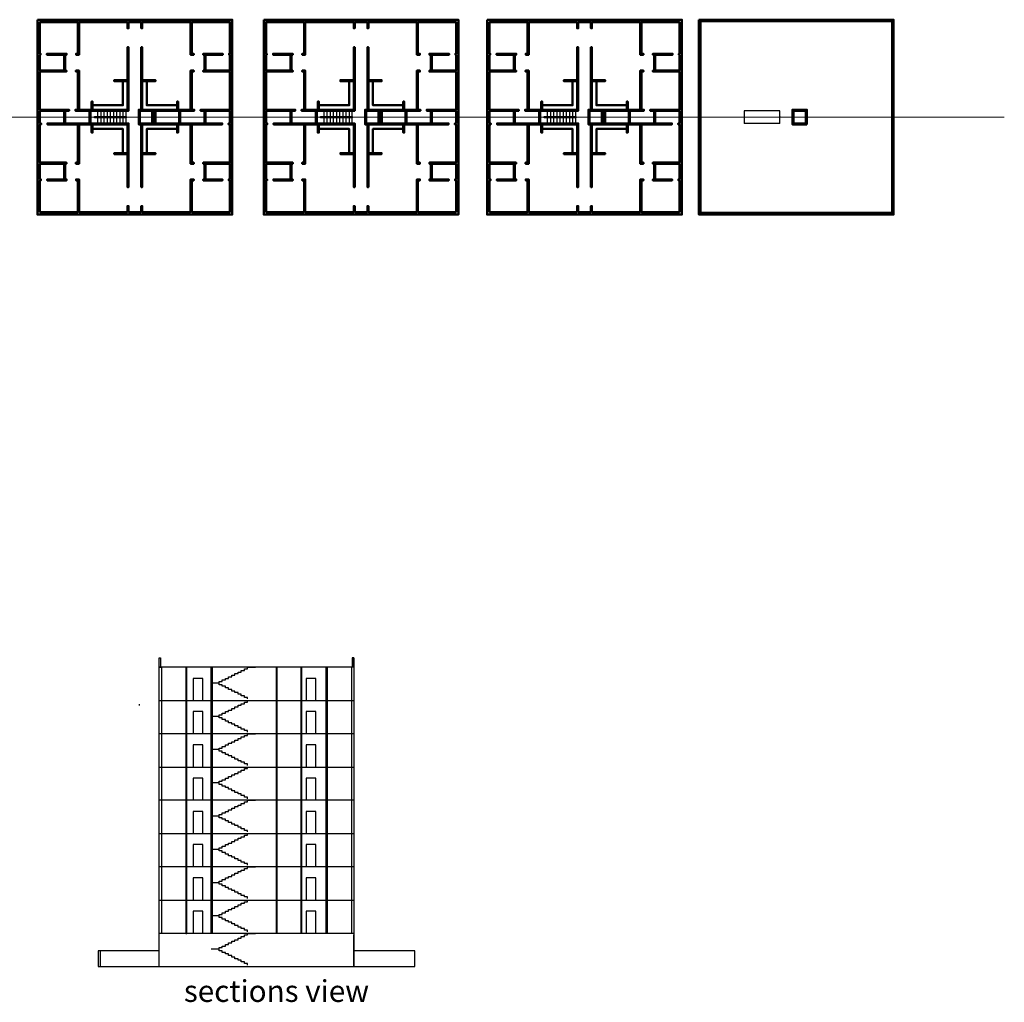
# Model space of a CAD drawing. Units: feet. Extents: x -1943 to 7856, y -1242 to 2749.
# Tile 2 of 2: x 4124 to 7856, y -1205 to 2518. Entities that reach past the tile are written whole.
import ezdxf

# ---------------------------------------------------------------- set-up
doc = ezdxf.new("R2010")
doc.units = ezdxf.units.FT
for name, color, linetype, lineweight in [('A-ANNO-SYMB', 1, 'Continuous', 18), ('A-ANNO-TEXT', 7, 'Continuous', 25), ('A-FLOR-STRS', 3, 'Continuous', 25), ('A-SECT', 7, 'Continuous', 25), ('A-WALL', 7, 'Continuous', 50)]:
    doc.layers.add(name, color=color, linetype=linetype, lineweight=lineweight)
doc.styles.get("Standard").update_dxf_attribs({"font": 'arial.ttf'})

# ---------------------------------------------------------------- blocks, each defined once
blk = doc.blocks.new('STAIR')
for p, q in [((-933.2, 2172.8), (-1068.1, 2172.8)), ((-1068.1, 2172.8), (-1068.1, 2124.8)), ((-1041.2, 2172.8), (-1041.2, 2151.4)), ((-1029.2, 2172.8), (-1029.2, 2151.4)), ((-1017.2, 2172.8), (-1017.2, 2151.4)), ((-1005.2, 2172.8), (-1005.2, 2151.4)), ((-993.2, 2172.8), (-993.2, 2151.4)), ((-981.2, 2172.8), (-981.2, 2151.4)), ((-969.2, 2172.8), (-969.2, 2151.4)), ((-957.2, 2172.8), (-957.2, 2151.4)), ((-945.2, 2172.8), (-945.2, 2151.4)), ((-1041.2, 2146.3), (-1041.2, 2124.8)), ((-1029.2, 2146.3), (-1029.2, 2124.8)), ((-1017.2, 2146.3), (-1017.2, 2124.8)), ((-1005.2, 2146.3), (-1005.2, 2124.8)), ((-993.2, 2146.3), (-993.2, 2124.8)), ((-981.2, 2146.3), (-981.2, 2124.8)), ((-969.2, 2146.3), (-969.2, 2124.8)), ((-957.2, 2146.3), (-957.2, 2124.8)), ((-933.2, 2124.8), (-1068.1, 2124.8))]:
    blk.add_line(p, q)
for points in [[(-933.2, 2124.8), (-933.2, 2172.8)], [(-945.2, 2146.3), (-945.2, 2124.8)]]:
    blk.add_lwpolyline(points)
for points in [[(-1053.2, 2151.4), (-933.2, 2151.4), (-933.2, 2146.3), (-1053.2, 2146.3)], [(-1052.2, 2150.4), (-934.2, 2150.4), (-934.2, 2147.3), (-1052.2, 2147.3)]]:
    blk.add_lwpolyline(points, close=True)

msp = doc.modelspace()

# ---------------------------------------------------------------- linework, layer by layer
at = {"layer": 'A-ANNO-SYMB'}
msp.add_line((-1942.9, 2148.8), (7856.1, 2148.8), dxfattribs=at)
at = {"layer": 'A-FLOR-STRS'}
for p, q in [((7005.2, 2172.8), (6870.3, 2172.8)), ((6870.3, 2172.8), (6870.3, 2124.8)), ((7005.2, 2124.8), (6870.3, 2124.8))]:
    msp.add_line(p, q, dxfattribs=at)
for points in [[(7005.2, 2124.8), (7005.2, 2172.8)], [(7005.2, 2151.4), (7005.2, 2148.8)]]:
    msp.add_lwpolyline(points, dxfattribs=at)
at = {"layer": 'A-SECT'}
for p, q in [((4652.5, 100.4), (4658.5, 100.4)), ((4652.5, -1069.6), (4652.5, 100.4)), ((4658.5, 100.4), (4658.5, 64.4)), ((5390.5, 100.4), (5384.5, 100.4)), ((5384.5, 100.4), (5384.5, 64.4)), ((5390.5, 64.4), (5390.5, 100.4)), ((5390.5, 100.4), (5390.5, -1069.6)), ((5390.5, 64.4), (4652.5, 64.4)), ((4652.5, 64.4), (4661.5, 64.4)), ((4661.5, 64.4), (4661.5, -943.6)), ((4753.5, 64.4), (4753.5, -943.6)), ((4757.5, -943.6), (4757.5, 64.4)), ((4849.5, -943.6), (4849.5, 64.4)), ((4849.5, 64.4), (4853.5, 64.4)), ((4853.5, 64.4), (4853.5, -943.6)), ((5100.7, 64.4), (5096.7, 64.4)), ((5096.7, 64.4), (5096.7, -943.6)), ((5100.7, -943.6), (5100.7, 64.4)), ((5189.5, 64.4), (5189.5, -943.6)), ((5193.5, -943.6), (5193.5, 64.4)), ((5285.5, -943.6), (5285.5, 64.4)), ((5289.5, 64.4), (5289.5, -943.6)), ((5381.5, 64.4), (5381.5, -943.6)), ((4652.5, -61.6), (5390.5, -61.6)), ((4577.1, -75.9, 316.9), (4577.1, -79.9, 316.9)), ((5390.5, -187.6), (4652.5, -187.6)), ((4652.5, -313.6), (5390.5, -313.6)), ((5390.5, -439.6), (4652.5, -439.6)), ((5390.5, -439.6), (4652.5, -439.6)), ((4652.5, -565.6), (5390.5, -565.6)), ((5390.5, -691.6), (4652.5, -691.6)), ((4652.5, -817.6), (5390.5, -817.6)), ((5390.5, -943.6), (4652.5, -943.6)), ((4753.5, -943.6), (4757.5, -943.6)), ((5390.5, -1069.6), (5390.5, -949.6)), ((4652.5, -1009.6), (4421.5, -1009.6)), ((4421.5, -1009.6), (4421.5, -1069.6)), ((4421.5, -1009.6), (4421.5, -1069.6)), ((4430.5, -1069.6), (4430.5, -1009.6)), ((5621.5, -1009.6), (5390.5, -1009.6)), ((5621.5, -1069.6), (5621.5, -1009.6)), ((4421.5, -1069.6), (5621.5, -1069.6))]:
    msp.add_line(p, q, dxfattribs=at)
for points in [[(4880.4, 4.4), (4880.4, 10.4), (4892.4, 10.4), (4892.4, 16.4), (4904.4, 16.4), (4904.4, 22.4), (4916.4, 22.4), (4916.4, 28.4), (4928.4, 28.4), (4928.4, 34.4), (4940.4, 34.4), (4940.4, 40.4), (4952.4, 40.4), (4952.4, 46.4), (4964.4, 46.4), (4964.4, 52.4), (4976.4, 52.4), (4976.4, 58.4), (4988.4, 58.4), (4988.4, 64.4), (5000.4, 64.4), (5018.5, 64.4)], [(4818.1, -61.6), (4818.1, 22.4), (4782.1, 22.4), (4782.1, -61.6)], [(4988.4, -55.6), (4988.4, -49.6), (4976.4, -49.6), (4976.4, -43.6), (4964.4, -43.6), (4964.4, -37.6), (4952.4, -37.6), (4952.4, -31.6), (4940.4, -31.6), (4940.4, -25.6), (4928.4, -25.6), (4928.4, -19.6), (4916.4, -19.6), (4916.4, -13.6), (4904.4, -13.6), (4904.4, -7.6), (4892.4, -7.6), (4892.4, -1.6), (4880.4, -1.6), (4880.4, 4.4), (4868.4, 4.4), (4850.4, 4.4)], [(5246.4, -61.6), (5246.4, 22.4), (5210.4, 22.4), (5210.4, -61.6)], [(4880.4, -121.6), (4880.4, -115.6), (4892.4, -115.6), (4892.4, -109.6), (4904.4, -109.6), (4904.4, -103.6), (4916.4, -103.6), (4916.4, -97.6), (4928.4, -97.6), (4928.4, -91.6), (4940.4, -91.6), (4940.4, -85.6), (4952.4, -85.6), (4952.4, -79.6), (4964.4, -79.6), (4964.4, -73.6), (4976.4, -73.6), (4976.4, -67.6), (4988.4, -67.6), (4988.4, -61.6), (5000.4, -61.6), (5018.5, -61.6)], [(4818.1, -187.6), (4818.1, -103.6), (4782.1, -103.6), (4782.1, -187.6)], [(5246.4, -187.6), (5246.4, -103.6), (5210.4, -103.6), (5210.4, -187.6)], [(4988.4, -181.6), (4988.4, -175.6), (4976.4, -175.6), (4976.4, -169.6), (4964.4, -169.6), (4964.4, -163.6), (4952.4, -163.6), (4952.4, -157.6), (4940.4, -157.6), (4940.4, -151.6), (4928.4, -151.6), (4928.4, -145.6), (4916.4, -145.6), (4916.4, -139.6), (4904.4, -139.6), (4904.4, -133.6), (4892.4, -133.6), (4892.4, -127.6), (4880.4, -127.6), (4880.4, -121.6), (4868.4, -121.6), (4850.4, -121.6)], [(4880.4, -247.6), (4880.4, -241.6), (4892.4, -241.6), (4892.4, -235.6), (4904.4, -235.6), (4904.4, -229.6), (4916.4, -229.6), (4916.4, -223.6), (4928.4, -223.6), (4928.4, -217.6), (4940.4, -217.6), (4940.4, -211.6), (4952.4, -211.6), (4952.4, -205.6), (4964.4, -205.6), (4964.4, -199.6), (4976.4, -199.6), (4976.4, -193.6), (4988.4, -193.6), (4988.4, -187.6), (5000.4, -187.6), (5018.5, -187.6)], [(4818.1, -313.6), (4818.1, -229.6), (4782.1, -229.6), (4782.1, -313.6)], [(4988.4, -307.6), (4988.4, -301.6), (4976.4, -301.6), (4976.4, -295.6), (4964.4, -295.6), (4964.4, -289.6), (4952.4, -289.6), (4952.4, -283.6), (4940.4, -283.6), (4940.4, -277.6), (4928.4, -277.6), (4928.4, -271.6), (4916.4, -271.6), (4916.4, -265.6), (4904.4, -265.6), (4904.4, -259.6), (4892.4, -259.6), (4892.4, -253.6), (4880.4, -253.6), (4880.4, -247.6), (4868.4, -247.6), (4850.4, -247.6)], [(5246.4, -313.6), (5246.4, -229.6), (5210.4, -229.6), (5210.4, -313.6)], [(4880.4, -373.6), (4880.4, -367.6), (4892.4, -367.6), (4892.4, -361.6), (4904.4, -361.6), (4904.4, -355.6), (4916.4, -355.6), (4916.4, -349.6), (4928.4, -349.6), (4928.4, -343.6), (4940.4, -343.6), (4940.4, -337.6), (4952.4, -337.6), (4952.4, -331.6), (4964.4, -331.6), (4964.4, -325.6), (4976.4, -325.6), (4976.4, -319.6), (4988.4, -319.6), (4988.4, -313.6), (5000.4, -313.6), (5018.5, -313.6)], [(4818.1, -439.6), (4818.1, -355.6), (4782.1, -355.6), (4782.1, -439.6)], [(5246.4, -439.6), (5246.4, -355.6), (5210.4, -355.6), (5210.4, -439.6)], [(4988.4, -433.6), (4988.4, -427.6), (4976.4, -427.6), (4976.4, -421.6), (4964.4, -421.6), (4964.4, -415.6), (4952.4, -415.6), (4952.4, -409.6), (4940.4, -409.6), (4940.4, -403.6), (4928.4, -403.6), (4928.4, -397.6), (4916.4, -397.6), (4916.4, -391.6), (4904.4, -391.6), (4904.4, -385.6), (4892.4, -385.6), (4892.4, -379.6), (4880.4, -379.6), (4880.4, -373.6), (4868.4, -373.6), (4850.4, -373.6)], [(4880.4, -499.6), (4880.4, -493.6), (4892.4, -493.6), (4892.4, -487.6), (4904.4, -487.6), (4904.4, -481.6), (4916.4, -481.6), (4916.4, -475.6), (4928.4, -475.6), (4928.4, -469.6), (4940.4, -469.6), (4940.4, -463.6), (4952.4, -463.6), (4952.4, -457.6), (4964.4, -457.6), (4964.4, -451.6), (4976.4, -451.6), (4976.4, -445.6), (4988.4, -445.6), (4988.4, -439.6), (5000.4, -439.6), (5018.5, -439.6)], [(4818.1, -565.6), (4818.1, -481.6), (4782.1, -481.6), (4782.1, -565.6)], [(5246.4, -565.6), (5246.4, -481.6), (5210.4, -481.6), (5210.4, -565.6)], [(4988.4, -559.6), (4988.4, -553.6), (4976.4, -553.6), (4976.4, -547.6), (4964.4, -547.6), (4964.4, -541.6), (4952.4, -541.6), (4952.4, -535.6), (4940.4, -535.6), (4940.4, -529.6), (4928.4, -529.6), (4928.4, -523.6), (4916.4, -523.6), (4916.4, -517.6), (4904.4, -517.6), (4904.4, -511.6), (4892.4, -511.6), (4892.4, -505.6), (4880.4, -505.6), (4880.4, -499.6), (4868.4, -499.6), (4850.4, -499.6)], [(4880.4, -625.6), (4880.4, -619.6), (4892.4, -619.6), (4892.4, -613.6), (4904.4, -613.6), (4904.4, -607.6), (4916.4, -607.6), (4916.4, -601.6), (4928.4, -601.6), (4928.4, -595.6), (4940.4, -595.6), (4940.4, -589.6), (4952.4, -589.6), (4952.4, -583.6), (4964.4, -583.6), (4964.4, -577.6), (4976.4, -577.6), (4976.4, -571.6), (4988.4, -571.6), (4988.4, -565.6), (5000.4, -565.6), (5018.5, -565.6)], [(4818.1, -691.6), (4818.1, -607.6), (4782.1, -607.6), (4782.1, -691.6)], [(4988.4, -685.6), (4988.4, -679.6), (4976.4, -679.6), (4976.4, -673.6), (4964.4, -673.6), (4964.4, -667.6), (4952.4, -667.6), (4952.4, -661.6), (4940.4, -661.6), (4940.4, -655.6), (4928.4, -655.6), (4928.4, -649.6), (4916.4, -649.6), (4916.4, -643.6), (4904.4, -643.6), (4904.4, -637.6), (4892.4, -637.6), (4892.4, -631.6), (4880.4, -631.6), (4880.4, -625.6), (4868.4, -625.6), (4850.4, -625.6)], [(5246.4, -691.6), (5246.4, -607.6), (5210.4, -607.6), (5210.4, -691.6)], [(4880.4, -751.6), (4880.4, -745.6), (4892.4, -745.6), (4892.4, -739.6), (4904.4, -739.6), (4904.4, -733.6), (4916.4, -733.6), (4916.4, -727.6), (4928.4, -727.6), (4928.4, -721.6), (4940.4, -721.6), (4940.4, -715.6), (4952.4, -715.6), (4952.4, -709.6), (4964.4, -709.6), (4964.4, -703.6), (4976.4, -703.6), (4976.4, -697.6), (4988.4, -697.6), (4988.4, -691.6), (5000.4, -691.6), (5018.5, -691.6)], [(4818.1, -817.6), (4818.1, -733.6), (4782.1, -733.6), (4782.1, -817.6)], [(5246.4, -817.6), (5246.4, -733.6), (5210.4, -733.6), (5210.4, -817.6)], [(4988.4, -811.6), (4988.4, -805.6), (4976.4, -805.6), (4976.4, -799.6), (4964.4, -799.6), (4964.4, -793.6), (4952.4, -793.6), (4952.4, -787.6), (4940.4, -787.6), (4940.4, -781.6), (4928.4, -781.6), (4928.4, -775.6), (4916.4, -775.6), (4916.4, -769.6), (4904.4, -769.6), (4904.4, -763.6), (4892.4, -763.6), (4892.4, -757.6), (4880.4, -757.6), (4880.4, -751.6), (4868.4, -751.6), (4850.4, -751.6)], [(4880.4, -877.6), (4880.4, -871.6), (4892.4, -871.6), (4892.4, -865.6), (4904.4, -865.6), (4904.4, -859.6), (4916.4, -859.6), (4916.4, -853.6), (4928.4, -853.6), (4928.4, -847.6), (4940.4, -847.6), (4940.4, -841.6), (4952.4, -841.6), (4952.4, -835.6), (4964.4, -835.6), (4964.4, -829.6), (4976.4, -829.6), (4976.4, -823.6), (4988.4, -823.6), (4988.4, -817.6), (5000.4, -817.6), (5018.5, -817.6)], [(4818.1, -943.6), (4818.1, -859.6), (4782.1, -859.6), (4782.1, -943.6)], [(4988.4, -937.6), (4988.4, -931.6), (4976.4, -931.6), (4976.4, -925.6), (4964.4, -925.6), (4964.4, -919.6), (4952.4, -919.6), (4952.4, -913.6), (4940.4, -913.6), (4940.4, -907.6), (4928.4, -907.6), (4928.4, -901.6), (4916.4, -901.6), (4916.4, -895.6), (4904.4, -895.6), (4904.4, -889.6), (4892.4, -889.6), (4892.4, -883.6), (4880.4, -883.6), (4880.4, -877.6), (4868.4, -877.6), (4850.4, -877.6)], [(5246.4, -943.6), (5246.4, -859.6), (5210.4, -859.6), (5210.4, -943.6)], [(4880.4, -1003.6), (4880.4, -997.6), (4892.4, -997.6), (4892.4, -991.6), (4904.4, -991.6), (4904.4, -985.6), (4916.4, -985.6), (4916.4, -979.6), (4928.4, -979.6), (4928.4, -973.6), (4940.4, -973.6), (4940.4, -967.6), (4952.4, -967.6), (4952.4, -961.6), (4964.4, -961.6), (4964.4, -955.6), (4976.4, -955.6), (4976.4, -949.6), (4988.4, -949.6), (4988.4, -943.6), (5000.4, -943.6), (5018.5, -943.6)], [(4988.4, -1063.6), (4988.4, -1057.6), (4976.4, -1057.6), (4976.4, -1051.6), (4964.4, -1051.6), (4964.4, -1045.6), (4952.4, -1045.6), (4952.4, -1039.6), (4940.4, -1039.6), (4940.4, -1033.6), (4928.4, -1033.6), (4928.4, -1027.6), (4916.4, -1027.6), (4916.4, -1021.6), (4904.4, -1021.6), (4904.4, -1015.6), (4892.4, -1015.6), (4892.4, -1009.6), (4880.4, -1009.6), (4880.4, -1003.6), (4868.4, -1003.6), (4850.4, -1003.6)]]:
    msp.add_lwpolyline(points, dxfattribs=at)
at = {"layer": 'A-WALL'}
for p, q in [((4639, 2288.8), (4639, 2288.8)), ((5496.3, 2288.8), (5496.3, 2288.8)), ((6343.2, 2288.8), (6343.2, 2288.8))]:
    msp.add_line(p, q, dxfattribs=at)
for points in [[(4191.9, 2517.8), (4191.9, 1779.8), (4929.9, 1779.8), (4929.9, 2517.8)], [(5049.2, 2517.8), (5049.2, 1779.8), (5787.2, 1779.8), (5787.2, 2517.8)], [(5896.1, 2517.8), (5896.1, 1779.8), (6634.1, 1779.8), (6634.1, 2517.8)], [(6698.6, 2517.8), (6698.6, 1779.8), (7436.6, 1779.8), (7436.6, 2517.8)], [(6704.6, 2511.8), (6704.6, 1785.8), (7430.6, 1785.8), (7430.6, 2511.8)], [(4630.5, 2120.8), (4575.8, 2120.8), (4575.8, 2176.8), (4630.5, 2176.8)], [(4626.5, 2124.8), (4579.8, 2124.8), (4579.8, 2172.8), (4626.5, 2172.8)], [(5487.8, 2120.8), (5433.2, 2120.8), (5433.2, 2176.8), (5487.8, 2176.8)], [(5483.8, 2124.8), (5437.2, 2124.8), (5437.2, 2172.8), (5483.8, 2172.8)], [(6334.7, 2120.8), (6280.1, 2120.8), (6280.1, 2176.8), (6334.7, 2176.8)], [(6330.7, 2124.8), (6284.1, 2124.8), (6284.1, 2172.8), (6330.7, 2172.8)], [(7107.8, 2120.8), (7053.2, 2120.8), (7053.2, 2176.8), (7107.8, 2176.8)], [(7103.8, 2124.8), (7057.2, 2124.8), (7057.2, 2172.8), (7103.8, 2172.8)]]:
    msp.add_lwpolyline(points, close=True, dxfattribs=at)
for points in [[(4732.9, 2124.8), (4824.9, 2124.8), (4824.9, 2172.8), (4810, 2172.8), (4810, 2176.8), (4920.9, 2176.8), (4920.9, 2321.3), (4820.1, 2321.3), (4820.1, 2325.3), (4824.9, 2325.3), (4824.9, 2384.8), (4819.8, 2384.8), (4819.8, 2388.8), (4894.3, 2388.8), (4894.3, 2384.8), (4828.9, 2384.8), (4828.9, 2325.3), (4920.9, 2325.3), (4920.9, 2384.8), (4918.3, 2384.8), (4918.3, 2388.8), (4920.9, 2388.8), (4920.9, 2508.8), (4776.4, 2508.8), (4776.4, 2388.8), (4783.8, 2388.8), (4783.8, 2384.8), (4772.4, 2384.8), (4772.4, 2508.8), (4588.9, 2508.8), (4588.9, 2485.7), (4584.9, 2485.7), (4584.9, 2508.8), (4536.9, 2508.8), (4536.9, 2485.7), (4532.9, 2485.7), (4532.9, 2508.8), (4349.4, 2508.8), (4349.4, 2384.8), (4337.9, 2384.8), (4337.9, 2388.8), (4345.4, 2388.8), (4345.4, 2508.8), (4200.9, 2508.8), (4200.9, 2388.8), (4203.4, 2388.8), (4203.4, 2384.8), (4200.9, 2384.8), (4200.9, 2325.3), (4292.9, 2325.3), (4292.9, 2384.8), (4227.4, 2384.8), (4227.4, 2388.8), (4301.9, 2388.8), (4301.9, 2384.8), (4296.9, 2384.8), (4296.9, 2325.3), (4301.7, 2325.3), (4301.7, 2321.3), (4200.9, 2321.3), (4200.9, 2176.8), (4311.8, 2176.8), (4311.8, 2172.8), (4296.9, 2172.8), (4296.9, 2124.8), (4388.9, 2124.8), (4388.9, 2172.8), (4388.9, 2124.8), (4388.9, 2172.8), (4335.8, 2172.8), (4335.8, 2176.8), (4345.4, 2176.8), (4345.4, 2321.3), (4337.7, 2321.3), (4337.7, 2325.3), (4349.4, 2325.3), (4349.4, 2176.8), (4396.9, 2176.8), (4396.9, 2207.4), (4400.9, 2207.4), (4400.9, 2176.8), (4532.9, 2176.8), (4532.9, 2284.8), (4482.8, 2284.8), (4482.8, 2288.8), (4532.9, 2288.8), (4532.9, 2413.7), (4536.9, 2413.7), (4536.9, 2172.8), (4392.9, 2172.8), (4392.9, 2124.8), (4536.9, 2124.8), (4536.9, 1884), (4532.9, 1884), (4532.9, 2008.8), (4482.8, 2008.8), (4482.8, 2012.8), (4532.9, 2012.8), (4532.9, 2120.8), (4400.9, 2120.8), (4400.9, 2090.3), (4396.9, 2090.3), (4396.9, 2120.8), (4349.4, 2120.8), (4349.4, 1972.3), (4337.7, 1972.3), (4337.7, 1976.3), (4345.4, 1976.3), (4345.4, 2120.8), (4229.4, 2120.8), (4229.4, 2124.8), (4292.9, 2124.8), (4292.9, 2172.8), (4200.9, 2172.8), (4200.9, 2124.8), (4205.4, 2124.8), (4205.4, 2120.8), (4200.9, 2120.8), (4200.9, 1976.3), (4301.7, 1976.3), (4301.7, 1972.3), (4296.9, 1972.3), (4296.9, 1912.8), (4301.9, 1912.8), (4301.9, 1908.8), (4228.8, 1908.8), (4228.8, 1912.8), (4292.9, 1912.8), (4292.9, 1972.3), (4200.9, 1972.3), (4200.9, 1912.8), (4204.8, 1912.8), (4204.8, 1908.8), (4200.9, 1908.8), (4200.9, 1788.8), (4345.4, 1788.8), (4345.4, 1908.8), (4337.9, 1908.8), (4337.9, 1912.8), (4349.4, 1912.8), (4349.4, 1788.8), (4532.9, 1788.8), (4532.9, 1812), (4536.9, 1812), (4536.9, 1788.8), (4584.9, 1788.8), (4584.9, 1812), (4588.9, 1812), (4588.9, 1788.8), (4772.4, 1788.8), (4772.4, 1912.8), (4783.8, 1912.8), (4783.8, 1908.8), (4776.4, 1908.8), (4776.4, 1788.8), (4920.9, 1788.8), (4920.9, 1908.8), (4917, 1908.8), (4917, 1912.8), (4920.9, 1912.8), (4920.9, 1972.3), (4828.9, 1972.3), (4828.9, 1912.8), (4893, 1912.8), (4893, 1908.8), (4819.8, 1908.8), (4819.8, 1912.8), (4824.9, 1912.8), (4824.9, 1972.3), (4820.1, 1972.3), (4820.1, 1976.3), (4920.9, 1976.3), (4920.9, 2120.8), (4916.4, 2120.8), (4916.4, 2124.8), (4920.9, 2124.8), (4920.9, 2172.8), (4828.9, 2172.8), (4828.9, 2124.8), (4892.4, 2124.8), (4892.4, 2120.8), (4776.4, 2120.8), (4776.4, 1976.3), (4784.1, 1976.3), (4784.1, 1972.3), (4772.4, 1972.3), (4772.4, 2120.8), (4724.9, 2120.8), (4724.9, 2090.3), (4720.9, 2090.3), (4720.9, 2120.8), (4588.9, 2120.8), (4588.9, 2012.8), (4639, 2012.8), (4639, 2008.8), (4588.9, 2008.8), (4588.9, 1884), (4584.9, 1884), (4584.9, 2124.8), (4635.5, 2124.8), (4635.5, 2172.8), (4584.9, 2172.8), (4584.9, 2413.7), (4588.9, 2413.7), (4588.9, 2288.8), (4639, 2288.8), (4639, 2284.8), (4588.9, 2284.8), (4588.9, 2176.8), (4720.9, 2176.8), (4720.9, 2207.4), (4724.9, 2207.4), (4724.9, 2176.8), (4772.4, 2176.8), (4772.4, 2325.3), (4784.1, 2325.3), (4784.1, 2321.3), (4776.4, 2321.3), (4776.4, 2176.8), (4786, 2176.8), (4786, 2172.8), (4732.9, 2172.8), (4732.9, 2124.8), (4732.9, 2172.8)], [(5590.2, 2124.8), (5682.2, 2124.8), (5682.2, 2172.8), (5667.3, 2172.8), (5667.3, 2176.8), (5778.2, 2176.8), (5778.2, 2321.3), (5677.4, 2321.3), (5677.4, 2325.3), (5682.2, 2325.3), (5682.2, 2384.8), (5677.2, 2384.8), (5677.2, 2388.8), (5751.7, 2388.8), (5751.7, 2384.8), (5686.2, 2384.8), (5686.2, 2325.3), (5778.2, 2325.3), (5778.2, 2384.8), (5775.7, 2384.8), (5775.7, 2388.8), (5778.2, 2388.8), (5778.2, 2508.8), (5633.7, 2508.8), (5633.7, 2388.8), (5641.2, 2388.8), (5641.2, 2384.8), (5629.7, 2384.8), (5629.7, 2508.8), (5446.2, 2508.8), (5446.2, 2485.7), (5442.2, 2485.7), (5442.2, 2508.8), (5394.2, 2508.8), (5394.2, 2485.7), (5390.2, 2485.7), (5390.2, 2508.8), (5206.7, 2508.8), (5206.7, 2384.8), (5195.3, 2384.8), (5195.3, 2388.8), (5202.7, 2388.8), (5202.7, 2508.8), (5058.2, 2508.8), (5058.2, 2388.8), (5060.8, 2388.8), (5060.8, 2384.8), (5058.2, 2384.8), (5058.2, 2325.3), (5150.2, 2325.3), (5150.2, 2384.8), (5084.8, 2384.8), (5084.8, 2388.8), (5159.3, 2388.8), (5159.3, 2384.8), (5154.2, 2384.8), (5154.2, 2325.3), (5159.1, 2325.3), (5159.1, 2321.3), (5058.2, 2321.3), (5058.2, 2176.8), (5169.1, 2176.8), (5169.1, 2172.8), (5154.2, 2172.8), (5154.2, 2124.8), (5246.2, 2124.8), (5246.2, 2172.8), (5246.2, 2124.8), (5246.2, 2172.8), (5193.1, 2172.8), (5193.1, 2176.8), (5202.7, 2176.8), (5202.7, 2321.3), (5195.1, 2321.3), (5195.1, 2325.3), (5206.7, 2325.3), (5206.7, 2176.8), (5254.2, 2176.8), (5254.2, 2207.4), (5258.2, 2207.4), (5258.2, 2176.8), (5390.2, 2176.8), (5390.2, 2284.8), (5340.2, 2284.8), (5340.2, 2288.8), (5390.2, 2288.8), (5390.2, 2413.7), (5394.2, 2413.7), (5394.2, 2172.8), (5250.2, 2172.8), (5250.2, 2124.8), (5394.2, 2124.8), (5394.2, 1884), (5390.2, 1884), (5390.2, 2008.8), (5340.2, 2008.8), (5340.2, 2012.8), (5390.2, 2012.8), (5390.2, 2120.8), (5258.2, 2120.8), (5258.2, 2090.3), (5254.2, 2090.3), (5254.2, 2120.8), (5206.7, 2120.8), (5206.7, 1972.3), (5195.1, 1972.3), (5195.1, 1976.3), (5202.7, 1976.3), (5202.7, 2120.8), (5086.7, 2120.8), (5086.7, 2124.8), (5150.2, 2124.8), (5150.2, 2172.8), (5058.2, 2172.8), (5058.2, 2124.8), (5062.7, 2124.8), (5062.7, 2120.8), (5058.2, 2120.8), (5058.2, 1976.3), (5159.1, 1976.3), (5159.1, 1972.3), (5154.2, 1972.3), (5154.2, 1912.8), (5159.3, 1912.8), (5159.3, 1908.8), (5086.1, 1908.8), (5086.1, 1912.8), (5150.2, 1912.8), (5150.2, 1972.3), (5058.2, 1972.3), (5058.2, 1912.8), (5062.1, 1912.8), (5062.1, 1908.8), (5058.2, 1908.8), (5058.2, 1788.8), (5202.7, 1788.8), (5202.7, 1908.8), (5195.3, 1908.8), (5195.3, 1912.8), (5206.7, 1912.8), (5206.7, 1788.8), (5390.2, 1788.8), (5390.2, 1812), (5394.2, 1812), (5394.2, 1788.8), (5442.2, 1788.8), (5442.2, 1812), (5446.2, 1812), (5446.2, 1788.8), (5629.7, 1788.8), (5629.7, 1912.8), (5641.2, 1912.8), (5641.2, 1908.8), (5633.7, 1908.8), (5633.7, 1788.8), (5778.2, 1788.8), (5778.2, 1908.8), (5774.3, 1908.8), (5774.3, 1912.8), (5778.2, 1912.8), (5778.2, 1972.3), (5686.2, 1972.3), (5686.2, 1912.8), (5750.3, 1912.8), (5750.3, 1908.8), (5677.2, 1908.8), (5677.2, 1912.8), (5682.2, 1912.8), (5682.2, 1972.3), (5677.4, 1972.3), (5677.4, 1976.3), (5778.2, 1976.3), (5778.2, 2120.8), (5773.7, 2120.8), (5773.7, 2124.8), (5778.2, 2124.8), (5778.2, 2172.8), (5686.2, 2172.8), (5686.2, 2124.8), (5749.7, 2124.8), (5749.7, 2120.8), (5633.7, 2120.8), (5633.7, 1976.3), (5641.4, 1976.3), (5641.4, 1972.3), (5629.7, 1972.3), (5629.7, 2120.8), (5582.2, 2120.8), (5582.2, 2090.3), (5578.2, 2090.3), (5578.2, 2120.8), (5446.2, 2120.8), (5446.2, 2012.8), (5496.3, 2012.8), (5496.3, 2008.8), (5446.2, 2008.8), (5446.2, 1884), (5442.2, 1884), (5442.2, 2124.8), (5492.8, 2124.8), (5492.8, 2172.8), (5442.2, 2172.8), (5442.2, 2413.7), (5446.2, 2413.7), (5446.2, 2288.8), (5496.3, 2288.8), (5496.3, 2284.8), (5446.2, 2284.8), (5446.2, 2176.8), (5578.2, 2176.8), (5578.2, 2207.4), (5582.2, 2207.4), (5582.2, 2176.8), (5629.7, 2176.8), (5629.7, 2325.3), (5641.4, 2325.3), (5641.4, 2321.3), (5633.7, 2321.3), (5633.7, 2176.8), (5643.3, 2176.8), (5643.3, 2172.8), (5590.2, 2172.8), (5590.2, 2124.8), (5590.2, 2172.8)], [(6437.1, 2124.8), (6529.1, 2124.8), (6529.1, 2172.8), (6514.2, 2172.8), (6514.2, 2176.8), (6625.1, 2176.8), (6625.1, 2321.3), (6524.3, 2321.3), (6524.3, 2325.3), (6529.1, 2325.3), (6529.1, 2384.8), (6524.1, 2384.8), (6524.1, 2388.8), (6598.6, 2388.8), (6598.6, 2384.8), (6533.1, 2384.8), (6533.1, 2325.3), (6625.1, 2325.3), (6625.1, 2384.8), (6622.6, 2384.8), (6622.6, 2388.8), (6625.1, 2388.8), (6625.1, 2508.8), (6480.6, 2508.8), (6480.6, 2388.8), (6488.1, 2388.8), (6488.1, 2384.8), (6476.6, 2384.8), (6476.6, 2508.8), (6293.1, 2508.8), (6293.1, 2485.7), (6289.1, 2485.7), (6289.1, 2508.8), (6241.1, 2508.8), (6241.1, 2485.7), (6237.1, 2485.7), (6237.1, 2508.8), (6053.6, 2508.8), (6053.6, 2384.8), (6042.2, 2384.8), (6042.2, 2388.8), (6049.6, 2388.8), (6049.6, 2508.8), (5905.1, 2508.8), (5905.1, 2388.8), (5907.7, 2388.8), (5907.7, 2384.8), (5905.1, 2384.8), (5905.1, 2325.3), (5997.1, 2325.3), (5997.1, 2384.8), (5931.7, 2384.8), (5931.7, 2388.8), (6006.2, 2388.8), (6006.2, 2384.8), (6001.1, 2384.8), (6001.1, 2325.3), (6006, 2325.3), (6006, 2321.3), (5905.1, 2321.3), (5905.1, 2176.8), (6016, 2176.8), (6016, 2172.8), (6001.1, 2172.8), (6001.1, 2124.8), (6093.1, 2124.8), (6093.1, 2172.8), (6093.1, 2124.8), (6093.1, 2172.8), (6040, 2172.8), (6040, 2176.8), (6049.6, 2176.8), (6049.6, 2321.3), (6042, 2321.3), (6042, 2325.3), (6053.6, 2325.3), (6053.6, 2176.8), (6101.1, 2176.8), (6101.1, 2207.4), (6105.1, 2207.4), (6105.1, 2176.8), (6237.1, 2176.8), (6237.1, 2284.8), (6187.1, 2284.8), (6187.1, 2288.8), (6237.1, 2288.8), (6237.1, 2413.7), (6241.1, 2413.7), (6241.1, 2172.8), (6097.1, 2172.8), (6097.1, 2124.8), (6241.1, 2124.8), (6241.1, 1884), (6237.1, 1884), (6237.1, 2008.8), (6187.1, 2008.8), (6187.1, 2012.8), (6237.1, 2012.8), (6237.1, 2120.8), (6105.1, 2120.8), (6105.1, 2090.3), (6101.1, 2090.3), (6101.1, 2120.8), (6053.6, 2120.8), (6053.6, 1972.3), (6042, 1972.3), (6042, 1976.3), (6049.6, 1976.3), (6049.6, 2120.8), (5933.6, 2120.8), (5933.6, 2124.8), (5997.1, 2124.8), (5997.1, 2172.8), (5905.1, 2172.8), (5905.1, 2124.8), (5909.6, 2124.8), (5909.6, 2120.8), (5905.1, 2120.8), (5905.1, 1976.3), (6006, 1976.3), (6006, 1972.3), (6001.1, 1972.3), (6001.1, 1912.8), (6006.2, 1912.8), (6006.2, 1908.8), (5933, 1908.8), (5933, 1912.8), (5997.1, 1912.8), (5997.1, 1972.3), (5905.1, 1972.3), (5905.1, 1912.8), (5909, 1912.8), (5909, 1908.8), (5905.1, 1908.8), (5905.1, 1788.8), (6049.6, 1788.8), (6049.6, 1908.8), (6042.2, 1908.8), (6042.2, 1912.8), (6053.6, 1912.8), (6053.6, 1788.8), (6237.1, 1788.8), (6237.1, 1812), (6241.1, 1812), (6241.1, 1788.8), (6289.1, 1788.8), (6289.1, 1812), (6293.1, 1812), (6293.1, 1788.8), (6476.6, 1788.8), (6476.6, 1912.8), (6488.1, 1912.8), (6488.1, 1908.8), (6480.6, 1908.8), (6480.6, 1788.8), (6625.1, 1788.8), (6625.1, 1908.8), (6621.2, 1908.8), (6621.2, 1912.8), (6625.1, 1912.8), (6625.1, 1972.3), (6533.1, 1972.3), (6533.1, 1912.8), (6597.2, 1912.8), (6597.2, 1908.8), (6524.1, 1908.8), (6524.1, 1912.8), (6529.1, 1912.8), (6529.1, 1972.3), (6524.3, 1972.3), (6524.3, 1976.3), (6625.1, 1976.3), (6625.1, 2120.8), (6620.6, 2120.8), (6620.6, 2124.8), (6625.1, 2124.8), (6625.1, 2172.8), (6533.1, 2172.8), (6533.1, 2124.8), (6596.6, 2124.8), (6596.6, 2120.8), (6480.6, 2120.8), (6480.6, 1976.3), (6488.3, 1976.3), (6488.3, 1972.3), (6476.6, 1972.3), (6476.6, 2120.8), (6429.1, 2120.8), (6429.1, 2090.3), (6425.1, 2090.3), (6425.1, 2120.8), (6293.1, 2120.8), (6293.1, 2012.8), (6343.2, 2012.8), (6343.2, 2008.8), (6293.1, 2008.8), (6293.1, 1884), (6289.1, 1884), (6289.1, 2124.8), (6339.7, 2124.8), (6339.7, 2172.8), (6289.1, 2172.8), (6289.1, 2413.7), (6293.1, 2413.7), (6293.1, 2288.8), (6343.2, 2288.8), (6343.2, 2284.8), (6293.1, 2284.8), (6293.1, 2176.8), (6425.1, 2176.8), (6425.1, 2207.4), (6429.1, 2207.4), (6429.1, 2176.8), (6476.6, 2176.8), (6476.6, 2325.3), (6488.3, 2325.3), (6488.3, 2321.3), (6480.6, 2321.3), (6480.6, 2176.8), (6490.2, 2176.8), (6490.2, 2172.8), (6437.1, 2172.8), (6437.1, 2124.8), (6437.1, 2172.8)], [(4400.9, 2193.8), (4515.9, 2193.8), (4515.9, 2284.8)], [(4720.9, 2193.8), (4605.9, 2193.8), (4605.9, 2284.8)], [(5258.2, 2193.8), (5373.2, 2193.8), (5373.2, 2284.8)], [(5578.2, 2193.8), (5463.2, 2193.8), (5463.2, 2284.8)], [(6105.1, 2193.8), (6220.2, 2193.8), (6220.2, 2284.8)], [(6425.1, 2193.8), (6310.1, 2193.8), (6310.1, 2284.8)], [(4728.9, 2124.8), (4639.5, 2124.8), (4639.5, 2172.8), (4728.9, 2172.8), (4728.9, 2124.8), (4728.9, 2172.8)], [(5586.2, 2124.8), (5496.8, 2124.8), (5496.8, 2172.8), (5586.2, 2172.8), (5586.2, 2124.8), (5586.2, 2172.8)], [(6433.1, 2124.8), (6343.7, 2124.8), (6343.7, 2172.8), (6433.1, 2172.8), (6433.1, 2124.8), (6433.1, 2172.8)], [(4400.9, 2103.9), (4515.9, 2103.9), (4515.9, 2012.8)], [(4720.9, 2103.9), (4605.9, 2103.9), (4605.9, 2012.8)], [(5258.2, 2103.9), (5373.2, 2103.9), (5373.2, 2012.8)], [(5578.2, 2103.9), (5463.2, 2103.9), (5463.2, 2012.8)], [(6105.1, 2103.9), (6220.2, 2103.9), (6220.2, 2012.8)], [(6425.1, 2103.9), (6310.1, 2103.9), (6310.1, 2012.8)]]:
    msp.add_lwpolyline(points, dxfattribs=at)

# ---------------------------------------------------------------- block references
at = {"layer": 'A-FLOR-STRS', "rotation": 0.0020692431570244}
for p in [(5461.1, 0), (6318.4, 0), (7165.3, 0)]:
    msp.add_blockref('STAIR', p, dxfattribs=at)

# ---------------------------------------------------------------- texts
at = {"layer": 'A-ANNO-TEXT', "insert": (4746.7, -1121), "char_height": 82.37, "attachment_point": 1}
msp.add_mtext_dynamic_manual_height_columns('sections view', width=36742.22, gutter_width=411.8, heights=[0], dxfattribs=at)

doc.saveas('drawing.dxf')
